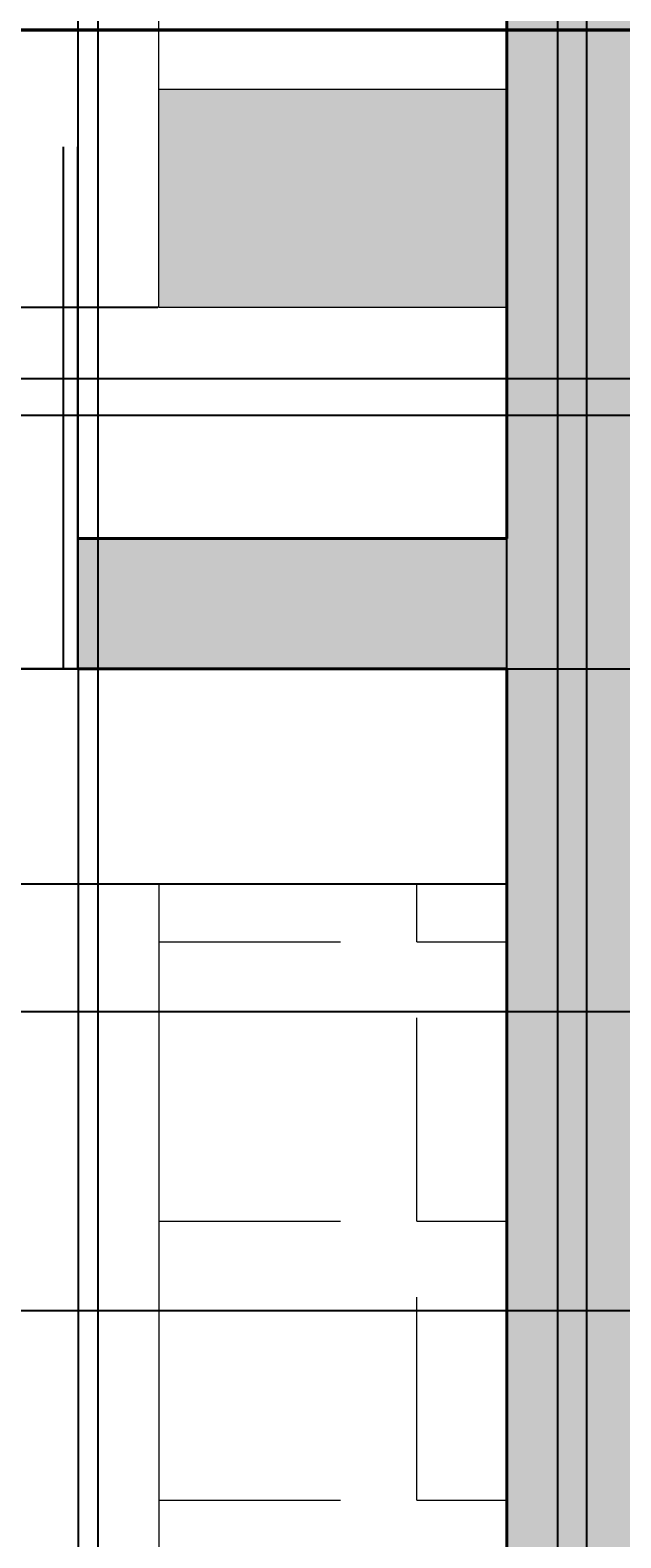
# Model space of a CAD drawing. Units: inches. Extents: x 818 to 1898, y 976 to 2364.
# Tile 25 of 96: x 1398 to 1439, y 1441 to 1545. Entities that reach past the tile are written whole.
import ezdxf

# ---------------------------------------------------------------- set-up
doc = ezdxf.new("R2010")
doc.units = ezdxf.units.IN
doc.header["$LTSCALE"] = 5
doc.header["$MEASUREMENT"] = 0
for name, color, linetype, lineweight in [('A-ANNO-DIMS', 2, 'Continuous', 18), ('A-DOOR', 3, 'Continuous', 25), ('A-FLOR-CASE', 8, 'Continuous', 18), ('A-FLOR-STRS', 7, 'Continuous', 25), ('A-FURN-PATT', 8, 'Continuous', 9), ('A-WALL', 7, 'Continuous', 40), ('C-PKNG', 8, 'Continuous', 18), ('C-PKNG-PATT', 9, 'Continuous', 9)]:
    doc.layers.add(name, color=color, linetype=linetype, lineweight=lineweight)
doc.layers.add('A-WALL-PATT', color=251, linetype='Continuous', lineweight=13, true_color=0x636466)
doc.styles.get("Standard").update_dxf_attribs({"font": 'arial.ttf'})
doc.dimstyles.get("Standard").update_dxf_attribs({"dimtxt": 0.18, "dimasz": 0.18, "dimexe": 0.18, "dimexo": 0.0625, "dimgap": 0.09, "dimtad": 0, "dimtih": 1, "dimtoh": 1, "dimdec": 4, "dimzin": 0, "dimdsep": 46, "dimtxsty": 'Standard', "dimcen": 0.09, "dimadec": 0, "dimazin": 0, "dimtfac": 1, "dimtdec": 4, "dimtofl": 0, "dimtmove": 0, "dimatfit": 3, "dimfxl": 1, "dimtolj": 1, "dimtzin": 0, "dimarcsym": 0})
pattern_1 = [(0, (0, 0), (0, 19.25), [14, -5.25]), (90, (0, 0), (-19.25, 1e-15), [14, -5.25])]

# ---------------------------------------------------------------- blocks, each defined once
blk = doc.blocks.new('*D61')
at = {"layer": 'A-ANNO-DIMS', "color": 0, "lineweight": -2, "ltscale": 5, "transparency": 16777216}
for p, q in [((1071.73, 1203.03), (1071.73, 2363.87)), ((1071.91, 2363.69), (1250.94, 2363.69)), ((1430.55, 2363.69), (1251.51, 2363.69)), ((1430.73, 1203.03), (1430.73, 2363.87))]:
    blk.add_line(p, q, dxfattribs=at)
at = {"layer": 'A-ANNO-DIMS', "color": 0, "ltscale": 5, "transparency": 16777216}
for points in [[(1071.91, 2363.72), (1071.91, 2363.66), (1071.73, 2363.69)], [(1430.55, 2363.72), (1430.55, 2363.66), (1430.73, 2363.69)]]:
    blk.add_solid(points, dxfattribs=at)
at = {"layer": 'Defpoints', "color": 0, "ltscale": 5, "transparency": 16777216}
for p in [(1430.73, 2363.69), (1071.73, 1202.96), (1430.73, 1202.96)]:
    blk.add_point(p, dxfattribs=at)
at = {"layer": 'A-ANNO-DIMS', "color": 0, "ltscale": 5, "transparency": 16777216, "insert": (1251.23, 2363.69), "char_height": 0.18, "attachment_point": 5}
blk.add_mtext('\\A1;359', dxfattribs=at)
blk = doc.blocks.new('*D64')
at = {"layer": 'A-ANNO-DIMS', "color": 0, "lineweight": -2, "ltscale": 5, "transparency": 16777216}
for p, q in [((1197.73, 1501.14), (1197.73, 2363.87)), ((1197.91, 2363.69), (1313.93, 2363.69)), ((1430.55, 2363.69), (1314.52, 2363.69)), ((1430.73, 1501.14), (1430.73, 2363.87))]:
    blk.add_line(p, q, dxfattribs=at)
at = {"layer": 'A-ANNO-DIMS', "color": 0, "ltscale": 5, "transparency": 16777216}
for points in [[(1197.91, 2363.72), (1197.91, 2363.66), (1197.73, 2363.69)], [(1430.55, 2363.72), (1430.55, 2363.66), (1430.73, 2363.69)]]:
    blk.add_solid(points, dxfattribs=at)
at = {"layer": 'Defpoints', "color": 0, "ltscale": 5, "transparency": 16777216}
for p in [(1430.73, 2363.69), (1197.73, 1501.08), (1430.73, 1501.08)]:
    blk.add_point(p, dxfattribs=at)
at = {"layer": 'A-ANNO-DIMS', "color": 0, "ltscale": 5, "transparency": 16777216, "insert": (1314.23, 2363.69), "char_height": 0.18, "attachment_point": 5}
blk.add_mtext('\\A1;233', dxfattribs=at)
blk = doc.blocks.new('*D99')
at = {"layer": 'A-ANNO-DIMS', "color": 0, "lineweight": -2, "ltscale": 5, "transparency": 16777216}
for p, q in [((1391.88, 1071.12), (1391.88, 2363.87)), ((1392.06, 2363.69), (1420.45, 2363.69)), ((1449.64, 2363.69), (1421.24, 2363.69)), ((1449.82, 1071.12), (1449.82, 2363.87))]:
    blk.add_line(p, q, dxfattribs=at)
at = {"layer": 'A-ANNO-DIMS', "color": 0, "ltscale": 5, "transparency": 16777216}
for points in [[(1392.06, 2363.72), (1392.06, 2363.66), (1391.88, 2363.69)], [(1449.64, 2363.72), (1449.64, 2363.66), (1449.82, 2363.69)]]:
    blk.add_solid(points, dxfattribs=at)
at = {"layer": 'Defpoints', "color": 0, "ltscale": 5, "transparency": 16777216}
for p in [(1449.82, 2363.69), (1391.88, 1071.06), (1449.82, 1071.06)]:
    blk.add_point(p, dxfattribs=at)
at = {"layer": 'A-ANNO-DIMS', "color": 0, "ltscale": 5, "transparency": 16777216, "insert": (1420.85, 2363.69), "char_height": 0.18, "attachment_point": 5}
blk.add_mtext('\\A1;57.94', dxfattribs=at)
blk = doc.blocks.new('*D116')
at = {"layer": 'A-ANNO-DIMS', "color": 0, "lineweight": -2, "ltscale": 5, "transparency": 16777216}
for p, q in [((1766.29, 1456.81), (818.03, 1456.81)), ((818.21, 1456.63), (818.21, 1417.41)), ((818.21, 1377.84), (818.21, 1417.05)), ((1766.29, 1377.66), (818.03, 1377.66))]:
    blk.add_line(p, q, dxfattribs=at)
at = {"layer": 'A-ANNO-DIMS', "color": 0, "ltscale": 5, "transparency": 16777216}
for points in [[(818.18, 1456.63), (818.24, 1456.63), (818.21, 1456.81)], [(818.18, 1377.84), (818.24, 1377.84), (818.21, 1377.66)]]:
    blk.add_solid(points, dxfattribs=at)
at = {"layer": 'Defpoints', "color": 0, "ltscale": 5, "transparency": 16777216}
for p in [(818.21, 1456.81), (1766.35, 1456.81), (1766.35, 1377.66)]:
    blk.add_point(p, dxfattribs=at)
at = {"layer": 'A-ANNO-DIMS', "color": 0, "ltscale": 5, "transparency": 16777216, "insert": (818.21, 1417.23), "char_height": 0.18, "attachment_point": 5}
blk.add_mtext('\\A1;79.15', dxfattribs=at)
blk = doc.blocks.new('*D117')
at = {"layer": 'A-ANNO-DIMS', "color": 0, "lineweight": -2, "ltscale": 5, "transparency": 16777216}
for p, q in [((1766.29, 1545.18), (818.03, 1545.18)), ((818.21, 1545), (818.21, 1501.18)), ((818.21, 1456.99), (818.21, 1500.81)), ((1766.29, 1456.81), (818.03, 1456.81))]:
    blk.add_line(p, q, dxfattribs=at)
at = {"layer": 'A-ANNO-DIMS', "color": 0, "ltscale": 5, "transparency": 16777216}
for points in [[(818.18, 1545), (818.24, 1545), (818.21, 1545.18)], [(818.18, 1456.99), (818.24, 1456.99), (818.21, 1456.81)]]:
    blk.add_solid(points, dxfattribs=at)
at = {"layer": 'Defpoints', "color": 0, "ltscale": 5, "transparency": 16777216}
for p in [(818.21, 1545.18), (1766.35, 1545.18), (1766.35, 1456.81)]:
    blk.add_point(p, dxfattribs=at)
at = {"layer": 'A-ANNO-DIMS', "color": 0, "ltscale": 5, "transparency": 16777216, "insert": (818.21, 1501), "char_height": 0.18, "attachment_point": 5}
blk.add_mtext('\\A1;88.37', dxfattribs=at)
blk = doc.blocks.new('*D159')
at = {"layer": 'A-ANNO-DIMS', "color": 0, "lineweight": -2, "ltscale": 5, "transparency": 16777216}
for p, q in [((1206.73, 1687.02), (1206.73, 975.66)), ((1463.73, 1687.02), (1463.73, 975.66)), ((1206.91, 975.84), (1334.93, 975.84)), ((1463.55, 975.84), (1335.52, 975.84))]:
    blk.add_line(p, q, dxfattribs=at)
at = {"layer": 'A-ANNO-DIMS', "color": 0, "ltscale": 5, "transparency": 16777216}
for points in [[(1206.91, 975.87), (1206.91, 975.81), (1206.73, 975.84)], [(1463.55, 975.87), (1463.55, 975.81), (1463.73, 975.84)]]:
    blk.add_solid(points, dxfattribs=at)
at = {"layer": 'Defpoints', "color": 0, "ltscale": 5, "transparency": 16777216}
for p in [(1206.73, 1687.08), (1463.73, 1687.08), (1463.73, 975.84)]:
    blk.add_point(p, dxfattribs=at)
at = {"layer": 'A-ANNO-DIMS', "color": 0, "ltscale": 5, "transparency": 16777216, "insert": (1335.23, 975.84), "char_height": 0.18, "attachment_point": 5}
blk.add_mtext('\\A1;257', dxfattribs=at)
blk = doc.blocks.new('*D163')
at = {"layer": 'A-ANNO-DIMS', "color": 0, "lineweight": -2, "ltscale": 5, "transparency": 16777216}
for p, q in [((1365.15, 1501.02), (1365.15, 975.66)), ((1401.15, 1501.02), (1401.15, 975.66)), ((1365.33, 975.84), (1382.93, 975.84)), ((1400.97, 975.84), (1383.37, 975.84))]:
    blk.add_line(p, q, dxfattribs=at)
at = {"layer": 'A-ANNO-DIMS', "color": 0, "ltscale": 5, "transparency": 16777216}
for points in [[(1365.33, 975.87), (1365.33, 975.81), (1365.15, 975.84)], [(1400.97, 975.87), (1400.97, 975.81), (1401.15, 975.84)]]:
    blk.add_solid(points, dxfattribs=at)
at = {"layer": 'Defpoints', "color": 0, "ltscale": 5, "transparency": 16777216}
for p in [(1365.15, 1501.08), (1401.15, 1501.08), (1401.15, 975.84)]:
    blk.add_point(p, dxfattribs=at)
at = {"layer": 'A-ANNO-DIMS', "color": 0, "ltscale": 5, "transparency": 16777216, "insert": (1383.15, 975.84), "char_height": 0.18, "attachment_point": 5}
blk.add_mtext('\\A1;36', dxfattribs=at)
blk = doc.blocks.new('*D166')
at = {"layer": 'A-ANNO-DIMS', "color": 0, "lineweight": -2, "ltscale": 5, "transparency": 16777216}
for p, q in [((1401.15, 1510.14), (1401.15, 2363.87)), ((1401.33, 2363.69), (1415.54, 2363.69)), ((1430.55, 2363.69), (1416.33, 2363.69)), ((1430.73, 1510.14), (1430.73, 2363.87))]:
    blk.add_line(p, q, dxfattribs=at)
at = {"layer": 'A-ANNO-DIMS', "color": 0, "ltscale": 5, "transparency": 16777216}
for points in [[(1401.33, 2363.72), (1401.33, 2363.66), (1401.15, 2363.69)], [(1430.55, 2363.72), (1430.55, 2363.66), (1430.73, 2363.69)]]:
    blk.add_solid(points, dxfattribs=at)
at = {"layer": 'Defpoints', "color": 0, "ltscale": 5, "transparency": 16777216}
for p in [(1430.73, 2363.69), (1401.15, 1510.08), (1430.73, 1510.08)]:
    blk.add_point(p, dxfattribs=at)
at = {"layer": 'A-ANNO-DIMS', "color": 0, "ltscale": 5, "transparency": 16777216, "insert": (1415.94, 2363.69), "char_height": 0.18, "attachment_point": 5}
blk.add_mtext('\\A1;29.58', dxfattribs=at)
blk = doc.blocks.new('*D167')
at = {"layer": 'A-ANNO-DIMS', "color": 0, "lineweight": -2, "ltscale": 5, "transparency": 16777216}
for p, q in [((1345.97, 1486.18), (1345.97, 975.66)), ((1430.73, 1486.18), (1430.73, 975.66)), ((1346.15, 975.84), (1387.95, 975.84)), ((1430.55, 975.84), (1388.74, 975.84))]:
    blk.add_line(p, q, dxfattribs=at)
at = {"layer": 'A-ANNO-DIMS', "color": 0, "ltscale": 5, "transparency": 16777216}
for points in [[(1346.15, 975.87), (1346.15, 975.81), (1345.97, 975.84)], [(1430.55, 975.87), (1430.55, 975.81), (1430.73, 975.84)]]:
    blk.add_solid(points, dxfattribs=at)
at = {"layer": 'Defpoints', "color": 0, "ltscale": 5, "transparency": 16777216}
for p in [(1345.97, 1486.24), (1430.73, 1486.24), (1430.73, 975.84)]:
    blk.add_point(p, dxfattribs=at)
at = {"layer": 'A-ANNO-DIMS', "color": 0, "ltscale": 5, "transparency": 16777216, "insert": (1388.35, 975.84), "char_height": 0.18, "attachment_point": 5}
blk.add_mtext('\\A1;84.76', dxfattribs=at)
blk = doc.blocks.new('*D168')
at = {"layer": 'A-ANNO-DIMS', "color": 0, "lineweight": -2, "ltscale": 5, "transparency": 16777216}
for p, q in [((1430.66, 1501.08), (818.03, 1501.08)), ((818.21, 1500.9), (818.21, 1493.84)), ((818.21, 1486.42), (818.21, 1493.48)), ((1430.66, 1486.24), (818.03, 1486.24))]:
    blk.add_line(p, q, dxfattribs=at)
at = {"layer": 'A-ANNO-DIMS', "color": 0, "ltscale": 5, "transparency": 16777216}
for points in [[(818.18, 1500.9), (818.24, 1500.9), (818.21, 1501.08)], [(818.18, 1486.42), (818.24, 1486.42), (818.21, 1486.24)]]:
    blk.add_solid(points, dxfattribs=at)
at = {"layer": 'Defpoints', "color": 0, "ltscale": 5, "transparency": 16777216}
for p in [(818.21, 1501.08), (1430.73, 1501.08), (1430.73, 1486.24)]:
    blk.add_point(p, dxfattribs=at)
at = {"layer": 'A-ANNO-DIMS', "color": 0, "ltscale": 5, "transparency": 16777216, "insert": (818.21, 1493.66), "char_height": 0.18, "attachment_point": 5}
blk.add_mtext('\\A1;14.84', dxfattribs=at)
blk = doc.blocks.new('*D170')
at = {"layer": 'A-ANNO-DIMS', "color": 0, "lineweight": -2, "ltscale": 5, "transparency": 16777216}
for p, q in [((1430.79, 1600.08), (1897.92, 1600.08)), ((1897.74, 1599.9), (1897.74, 1550.76)), ((1897.74, 1501.26), (1897.74, 1550.4)), ((1430.79, 1501.08), (1897.92, 1501.08))]:
    blk.add_line(p, q, dxfattribs=at)
at = {"layer": 'A-ANNO-DIMS', "color": 0, "ltscale": 5, "transparency": 16777216}
for points in [[(1897.71, 1599.9), (1897.77, 1599.9), (1897.74, 1600.08)], [(1897.71, 1501.26), (1897.77, 1501.26), (1897.74, 1501.08)]]:
    blk.add_solid(points, dxfattribs=at)
at = {"layer": 'Defpoints', "color": 0, "ltscale": 5, "transparency": 16777216}
for p in [(1430.73, 1600.08), (1897.74, 1600.08), (1430.73, 1501.08)]:
    blk.add_point(p, dxfattribs=at)
at = {"layer": 'A-ANNO-DIMS', "color": 0, "ltscale": 5, "transparency": 16777216, "insert": (1897.74, 1550.58), "char_height": 0.18, "attachment_point": 5}
blk.add_mtext('\\A1;99', dxfattribs=at)
blk = doc.blocks.new('*D187')
at = {"layer": 'A-ANNO-DIMS', "color": 0, "lineweight": -2, "ltscale": 5, "transparency": 16777216}
for p, q in [((1705.66, 1545.08), (818.03, 1545.08)), ((818.21, 1544.9), (818.21, 1533.26)), ((818.21, 1521.26), (818.21, 1532.9)), ((1705.66, 1521.08), (818.03, 1521.08))]:
    blk.add_line(p, q, dxfattribs=at)
at = {"layer": 'A-ANNO-DIMS', "color": 0, "ltscale": 5, "transparency": 16777216}
for points in [[(818.18, 1544.9), (818.24, 1544.9), (818.21, 1545.08)], [(818.18, 1521.26), (818.24, 1521.26), (818.21, 1521.08)]]:
    blk.add_solid(points, dxfattribs=at)
at = {"layer": 'Defpoints', "color": 0, "ltscale": 5, "transparency": 16777216}
for p in [(818.21, 1545.08), (1705.73, 1545.08), (1705.73, 1521.08)]:
    blk.add_point(p, dxfattribs=at)
at = {"layer": 'A-ANNO-DIMS', "color": 0, "ltscale": 5, "transparency": 16777216, "insert": (818.21, 1533.08), "char_height": 0.18, "attachment_point": 5}
blk.add_mtext('\\A1;24', dxfattribs=at)
blk = doc.blocks.new('*D191')
at = {"layer": 'A-ANNO-DIMS', "color": 0, "lineweight": -2, "ltscale": 5, "transparency": 16777216}
for p, q in [((1434.23, 1409.11), (1434.23, 2363.87)), ((1434.41, 2363.69), (1435.08, 2363.69)), ((1436.05, 2363.69), (1435.37, 2363.69)), ((1436.23, 1409.11), (1436.23, 2363.87))]:
    blk.add_line(p, q, dxfattribs=at)
at = {"layer": 'A-ANNO-DIMS', "color": 0, "ltscale": 5, "transparency": 16777216}
for points in [[(1434.41, 2363.72), (1434.41, 2363.66), (1434.23, 2363.69)], [(1436.05, 2363.72), (1436.05, 2363.66), (1436.23, 2363.69)]]:
    blk.add_solid(points, dxfattribs=at)
at = {"layer": 'Defpoints', "color": 0, "ltscale": 5, "transparency": 16777216}
for p in [(1436.23, 2363.69), (1434.23, 1409.05), (1436.23, 1409.05)]:
    blk.add_point(p, dxfattribs=at)
at = {"layer": 'A-ANNO-DIMS', "color": 0, "ltscale": 5, "transparency": 16777216, "insert": (1435.23, 2363.69), "char_height": 0.18, "attachment_point": 5}
blk.add_mtext('\\A1;2', dxfattribs=at)
blk = doc.blocks.new('*D198')
at = {"layer": 'A-ANNO-DIMS', "color": 0, "lineweight": -2, "ltscale": 5, "transparency": 16777216}
for p, q in [((1741.84, 1545.02), (1741.84, 975.66)), ((1430.73, 1346.02), (1430.73, 975.66)), ((1430.91, 975.84), (1585.91, 975.84)), ((1741.66, 975.84), (1586.66, 975.84))]:
    blk.add_line(p, q, dxfattribs=at)
at = {"layer": 'A-ANNO-DIMS', "color": 0, "ltscale": 5, "transparency": 16777216}
for points in [[(1430.91, 975.87), (1430.91, 975.81), (1430.73, 975.84)], [(1741.66, 975.87), (1741.66, 975.81), (1741.84, 975.84)]]:
    blk.add_solid(points, dxfattribs=at)
at = {"layer": 'Defpoints', "color": 0, "ltscale": 5, "transparency": 16777216}
for p in [(1741.84, 1545.08), (1430.73, 1346.08), (1741.84, 975.84)]:
    blk.add_point(p, dxfattribs=at)
at = {"layer": 'A-ANNO-DIMS', "color": 0, "ltscale": 5, "transparency": 16777216, "insert": (1586.28, 975.84), "char_height": 0.18, "attachment_point": 5}
blk.add_mtext('\\A1;311.1', dxfattribs=at)
blk = doc.blocks.new('*D201')
at = {"layer": 'A-ANNO-DIMS', "color": 0, "lineweight": -2, "ltscale": 5, "transparency": 16777216}
for p, q in [((1678.27, 1518.56), (818.03, 1518.56)), ((818.21, 1518.38), (818.21, 1498.18)), ((818.21, 1477.61), (818.21, 1497.81)), ((1678.27, 1477.43), (818.03, 1477.43))]:
    blk.add_line(p, q, dxfattribs=at)
at = {"layer": 'A-ANNO-DIMS', "color": 0, "ltscale": 5, "transparency": 16777216}
for points in [[(818.18, 1518.38), (818.24, 1518.38), (818.21, 1518.56)], [(818.18, 1477.61), (818.24, 1477.61), (818.21, 1477.43)]]:
    blk.add_solid(points, dxfattribs=at)
at = {"layer": 'Defpoints', "color": 0, "ltscale": 5, "transparency": 16777216}
for p in [(818.21, 1518.56), (1678.33, 1518.56), (1678.33, 1477.43)]:
    blk.add_point(p, dxfattribs=at)
at = {"layer": 'A-ANNO-DIMS', "color": 0, "ltscale": 5, "transparency": 16777216, "insert": (818.21, 1497.99), "char_height": 0.18, "attachment_point": 5}
blk.add_mtext('\\A1;41.135', dxfattribs=at)
blk = doc.blocks.new('*D231')
at = {"layer": 'A-ANNO-DIMS', "color": 0, "lineweight": -2, "ltscale": 5, "transparency": 16777216}
for p, q in [((1303.93, 1952.98), (1303.93, 975.66)), ((1402.52, 1952.98), (1402.52, 975.66)), ((1304.11, 975.84), (1352.83, 975.84)), ((1402.34, 975.84), (1353.62, 975.84))]:
    blk.add_line(p, q, dxfattribs=at)
at = {"layer": 'A-ANNO-DIMS', "color": 0, "ltscale": 5, "transparency": 16777216}
for points in [[(1304.11, 975.87), (1304.11, 975.81), (1303.93, 975.84)], [(1402.34, 975.87), (1402.34, 975.81), (1402.52, 975.84)]]:
    blk.add_solid(points, dxfattribs=at)
at = {"layer": 'Defpoints', "color": 0, "ltscale": 5, "transparency": 16777216}
for p in [(1303.93, 1953.04), (1402.52, 1953.04), (1402.52, 975.84)]:
    blk.add_point(p, dxfattribs=at)
at = {"layer": 'A-ANNO-DIMS', "color": 0, "ltscale": 5, "transparency": 16777216, "insert": (1353.22, 975.84), "char_height": 0.18, "attachment_point": 5}
blk.add_mtext('\\A1;98.59', dxfattribs=at)
blk = doc.blocks.new('*D272')
at = {"layer": 'A-ANNO-DIMS', "color": 0, "lineweight": -2, "ltscale": 5, "transparency": 16777216}
for p, q in [((1406.66, 1587.42), (818.03, 1587.42)), ((818.21, 1587.24), (818.21, 1556.89)), ((818.21, 1526.18), (818.21, 1556.52)), ((1406.66, 1526), (818.03, 1526))]:
    blk.add_line(p, q, dxfattribs=at)
at = {"layer": 'A-ANNO-DIMS', "color": 0, "ltscale": 5, "transparency": 16777216}
for points in [[(818.18, 1587.24), (818.24, 1587.24), (818.21, 1587.42)], [(818.18, 1526.18), (818.24, 1526.18), (818.21, 1526)]]:
    blk.add_solid(points, dxfattribs=at)
at = {"layer": 'Defpoints', "color": 0, "ltscale": 5, "transparency": 16777216}
for p in [(818.21, 1587.42), (1406.73, 1587.42), (1406.73, 1526)]:
    blk.add_point(p, dxfattribs=at)
at = {"layer": 'A-ANNO-DIMS', "color": 0, "ltscale": 5, "transparency": 16777216, "insert": (818.21, 1556.71), "char_height": 0.18, "attachment_point": 5}
blk.add_mtext('\\A1;61.42', dxfattribs=at)

msp = doc.modelspace()

# ---------------------------------------------------------------- hatches: boundary and pattern name
at = {"layer": 'A-FURN-PATT', "ltscale": 5}
h = msp.add_hatch(color=256, dxfattribs=at)
h.dxf.hatch_style = 1
h.paths.add_polyline_path([(1336.7936, 1953.0408), (1314.2595, 1953.0408), (1314.2595, 1941.0096), (1336.7936, 1941.0096)])
h.paths.add_polyline_path([(1338.9915, 1941.0096), (1336.7936, 1941.0096), (1336.7936, 1937.7177), (1314.2595, 1937.7177), (1314.2595, 1941.0096), (1310.9077, 1941.0096), (1310.9077, 1935.2252), (1338.9915, 1935.2252)])
h.paths.add_polyline_path([(1336.7936, 1941.0096), (1314.2595, 1941.0096), (1314.2595, 1937.7177), (1336.7936, 1937.7177)], flags=17)
h.paths.add_polyline_path([(1367.9307, 1959.6079), (1345.3966, 1959.6079), (1345.3966, 1941.0096), (1367.9307, 1941.0096)])
h.paths.add_polyline_path([(1398.8475, 1953.0408), (1376.3134, 1953.0408), (1376.3134, 1952.6393), (1390.1242, 1941.0096), (1398.8475, 1941.0096)])
h.paths.add_polyline_path([(1376.3134, 1952.6393), (1376.3134, 1941.0096), (1390.1242, 1941.0096)], flags=17)
h.paths.add_polyline_path([(1370.1286, 1941.0096), (1367.9307, 1941.0096), (1367.9307, 1937.7177), (1345.3966, 1937.7177), (1345.3966, 1941.0096), (1342.0448, 1941.0096), (1342.0448, 1935.2252), (1370.1286, 1935.2252)])
h.paths.add_polyline_path([(1367.9307, 1941.0096), (1345.3966, 1941.0096), (1345.3966, 1937.7177), (1367.9307, 1937.7177)], flags=17)
h.paths.add_polyline_path([(1390.1242, 1941.0096), (1376.3134, 1941.0096), (1376.3134, 1937.7177), (1394.0336, 1937.7177)], flags=17)
h.paths.add_polyline_path([(1394.0336, 1937.7177), (1376.3134, 1937.7177), (1376.3134, 1941.0096), (1372.9616, 1941.0096), (1372.9616, 1935.2252), (1396.9935, 1935.2252)])
h.paths.add_polyline_path([(1398.8475, 1941.0096), (1390.1242, 1941.0096), (1394.0336, 1937.7177), (1398.8475, 1937.7177)])
h.paths.add_polyline_path([(1401.0455, 1941.0096), (1398.8475, 1941.0096), (1398.8475, 1937.7177), (1394.0336, 1937.7177), (1396.9935, 1935.2252), (1401.0455, 1935.2252)])
h.paths.add_polyline_path([(1336.7936, 2020.4229), (1314.2595, 2020.4229), (1314.2595, 2008.3917), (1336.7936, 2008.3917)])
h.paths.add_polyline_path([(1336.7936, 2023.7149), (1314.2595, 2023.7149), (1314.2595, 2020.4229), (1336.7936, 2020.4229)], flags=17)
h.paths.add_polyline_path([(1338.9915, 2026.2074), (1310.9077, 2026.2074), (1310.9077, 2020.4229), (1314.2595, 2020.4229), (1314.2595, 2023.7149), (1336.7936, 2023.7149), (1336.7936, 2020.4229), (1338.9915, 2020.4229)])
h.paths.add_polyline_path([(1367.9307, 2023.7149), (1345.3966, 2023.7149), (1345.3966, 2020.4229), (1367.9307, 2020.4229)], flags=17)
h.paths.add_polyline_path([(1370.1286, 2026.2074), (1342.0448, 2026.2074), (1342.0448, 2020.4229), (1345.3966, 2020.4229), (1345.3966, 2023.7149), (1367.9307, 2023.7149), (1367.9307, 2020.4229), (1370.1286, 2020.4229)])
h.paths.add_polyline_path([(1367.9307, 2020.4229), (1345.3966, 2020.4229), (1345.3966, 2008.3917), (1367.9307, 2008.3917)])
h.paths.add_polyline_path([(1398.8475, 2020.4229), (1388.1824, 2020.4229), (1376.3134, 2010.4284), (1376.3134, 2008.3917), (1398.8475, 2008.3917)])
h.paths.add_polyline_path([(1392.0918, 2023.7149), (1376.3134, 2023.7149), (1376.3134, 2020.4229), (1388.1824, 2020.4229)], flags=17)
h.paths.add_polyline_path([(1388.1824, 2020.4229), (1376.3134, 2020.4229), (1376.3134, 2010.4284)], flags=17)
h.paths.add_polyline_path([(1395.0518, 2026.2074), (1372.9616, 2026.2074), (1372.9616, 2020.4229), (1376.3134, 2020.4229), (1376.3134, 2023.7149), (1392.0918, 2023.7149)])
h.paths.add_polyline_path([(1398.8475, 2023.7149), (1392.0918, 2023.7149), (1388.1824, 2020.4229), (1398.8475, 2020.4229)])
h.paths.add_polyline_path([(1401.0455, 2026.2074), (1395.0518, 2026.2074), (1392.0918, 2023.7149), (1398.8475, 2023.7149), (1398.8475, 2020.4229), (1401.0455, 2020.4229)])
h.paths.add_polyline_path([(1327.0339, 1897.8663), (1311.025, 1897.8663), (1311.025, 1876.0782), (1327.0339, 1876.0782)])
h.paths.add_polyline_path([(1377.7791, 1897.8663), (1359.9579, 1897.8663), (1359.9579, 1876.0782), (1377.7791, 1876.0782)])
h.paths.add_polyline_path([(1430.7251, 1541.0439), (1406.7251, 1541.0439), (1406.7251, 1525.9965), (1430.7251, 1525.9965)])
h.paths.add_polyline_path([(1430.7251, 1587.4164), (1406.7251, 1587.4164), (1406.7251, 1570.9187), (1430.7251, 1570.9187)])
at = {"layer": 'A-WALL-PATT', "ltscale": 5}
h = msp.add_hatch(color=256, dxfattribs=at)
h.dxf.hatch_style = 1
h.paths.add_polyline_path([(1206.7251, 1687.0782), (1206.7251, 1700.0782), (1197.7251, 1700.0782), (1197.7251, 1501.0782), (1206.7251, 1501.0782), (1206.7251, 1510.0782)])
h.paths.add_polyline_path([(1197.7251, 1590.7585), (1173.7252, 1590.7585), (1173.7252, 1586.7585), (1197.7251, 1586.7585)])
h.paths.add_polyline_path([(1197.7251, 1534.6024), (1173.7252, 1534.6024), (1173.7252, 1530.6024), (1197.7251, 1530.6024)])
h.paths.add_polyline_path([(1365.1463, 1510.0782), (1283.8183, 1510.0782), (1283.8183, 1501.0782), (1365.1463, 1501.0782)])
h.paths.add_polyline_path([(1439.7252, 1591.0782), (1441.7252, 1591.0782), (1441.7252, 1600.0782), (1430.7251, 1600.0782), (1430.7251, 1510.0782), (1406.7251, 1510.0782), (1401.1463, 1510.0782), (1401.1463, 1501.0782), (1430.7251, 1501.0782), (1430.7251, 1486.2383), (1430.7251, 1409.0522), (1439.7252, 1409.0522)])
at = {"layer": 'C-PKNG-PATT', "ltscale": 5}
h = msp.add_hatch(dxfattribs=at)
h.set_pattern_fill('ANGLE', color=256, scale=70)
h.set_pattern_definition(pattern_1)
h.paths.add_polyline_path([(1430.7251, 1211.9642), (1430.7251, 1486.2383), (1406.7251, 1486.2383), (1406.7251, 1235.9642), (1116.1882, 1235.9642), (1116.1882, 1485.2035), (1345.9651, 1485.2035), (1345.9651, 1501.0782), (1206.7251, 1501.0782), (1197.7251, 1501.0782), (1083.7252, 1501.0782), (1083.7252, 1485.2035), (1083.7252, 1211.9642)])
h = msp.add_hatch(dxfattribs=at)
h.set_pattern_fill('ANGLE', color=256, scale=70)
h.set_pattern_definition(pattern_1)
h.paths.add_polyline_path([(1116.1882, 1485.2035), (1345.9651, 1485.2035), (1345.9651, 1501.0782), (1206.7251, 1501.0782), (1197.7251, 1501.0782), (1083.7252, 1501.0782), (1083.7252, 1485.2035), (1083.7252, 1211.9642), (1430.7251, 1211.9642), (1430.7251, 1271.1621), (1430.7251, 1290.0782), (1430.7251, 1346.0782), (1430.7251, 1486.2383), (1406.7251, 1486.2383), (1406.7251, 1235.9642), (1116.1882, 1235.9642)])

# ---------------------------------------------------------------- linework, layer by layer
at = {"layer": 'A-DOOR'}
for p, q in [((1400.1463, 1501.0782), (1400.1463, 1537.0782)), ((1401.1463, 1501.0782), (1401.1463, 1537.0782)), ((1401.1463, 1510.0782), (1401.1463, 1501.0782))]:
    msp.add_line(p, q, dxfattribs=at)
at = {"layer": 'A-FLOR-CASE'}
for p, q in [((1406.7251, 1525.9965), (1406.7251, 1587.4164)), ((1430.7251, 1525.9965), (1406.7251, 1525.9965)), ((1430.7251, 1510.0782), (1406.7251, 1510.0782))]:
    msp.add_line(p, q, dxfattribs=at)
msp.add_lwpolyline([(1406.7251, 1570.9187), (1430.7251, 1570.9187), (1430.7251, 1541.0439), (1406.7251, 1541.0439)], close=True, dxfattribs=at)
at = {"layer": 'A-FLOR-STRS'}
msp.add_lwpolyline([(1345.9651, 1501.0782), (1430.7251, 1501.0782), (1430.7251, 1486.2383), (1345.9651, 1486.2383)], close=True, dxfattribs=at)
at = {"layer": 'A-WALL'}
for p, q in [((1430.7251, 1600.0782), (1430.7251, 1510.0782)), ((1401.1463, 1510.0782), (1430.7251, 1510.0782)), ((1401.1463, 1501.0782), (1430.7251, 1501.0782)), ((1430.7251, 1501.0782), (1430.7251, 1346.0782))]:
    msp.add_line(p, q, dxfattribs=at)
at = {"layer": 'C-PKNG'}
msp.add_line((1406.7251, 1486.2383), (1406.7251, 1235.9642), dxfattribs=at)

# ---------------------------------------------------------------- dimensions: what is measured, and where the dimension line sits
at = {"layer": 'A-ANNO-DIMS', "ltscale": 5}
for base, p1, p2, override, picture, middle in [((1430.7251, 2363.6929), (1071.7251, 1202.9642), (1430.7251, 1202.9642), {"dimdec": 0, "dimlfac": 1, "dimrnd": 0, "dimzin": 0, "dimdsep": 46, "dimlunit": 2}, '*D61', (1251.2251, 2363.6929)), ((1430.7251, 2363.6929), (1197.7251, 1501.0782), (1430.7251, 1501.0782), {"dimdec": 0, "dimlfac": 1, "dimrnd": 0, "dimzin": 0, "dimdsep": 46, "dimlunit": 2}, '*D64', (1314.2251, 2363.6929)), ((1449.8196, 2363.6929), (1391.8757, 1071.0552), (1449.8196, 1071.0552), {"dimdec": 2, "dimlfac": 1, "dimrnd": 0, "dimzin": 0, "dimdsep": 46, "dimlunit": 2}, '*D99', (1420.8477, 2363.6929)), ((1430.7251, 2363.6929), (1401.1463, 1510.0782), (1430.7251, 1510.0782), {"dimdec": 2, "dimlfac": 1, "dimrnd": 0, "dimzin": 0, "dimdsep": 46, "dimlunit": 2}, '*D166', (1415.9357, 2363.6929)), ((1436.2251, 2363.6929), (1434.2251, 1409.0522), (1436.2251, 1409.0522), {"dimdec": 0, "dimlfac": 1, "dimrnd": 0, "dimzin": 0, "dimdsep": 46, "dimlunit": 2}, '*D191', (1435.2251, 2363.6929)), ((1402.518, 975.8433), (1303.9314, 1953.0408), (1402.518, 1953.0408), {"dimdec": 2, "dimlfac": 1, "dimrnd": 0, "dimzin": 0, "dimdsep": 46, "dimlunit": 2}, '*D231', (1353.2247, 975.8433)), ((1463.7251, 975.8433), (1206.7251, 1687.0782), (1463.7251, 1687.0782), {"dimdec": 0, "dimlfac": 1, "dimrnd": 0, "dimzin": 0, "dimdsep": 46, "dimlunit": 2}, '*D159', (1335.2251, 975.8433)), ((1741.8409, 975.8433), (1430.7251, 1346.0782), (1741.8409, 1545.0782), {"dimdec": 1, "dimlfac": 1, "dimrnd": 0, "dimzin": 0, "dimdsep": 46, "dimlunit": 2}, '*D198', (1586.283, 975.8433)), ((1401.1463, 975.8433), (1365.1463, 1501.0782), (1401.1463, 1501.0782), {"dimdec": 0, "dimlfac": 1, "dimrnd": 0, "dimzin": 0, "dimdsep": 46, "dimlunit": 2}, '*D163', (1383.1463, 975.8433)), ((1430.7251, 975.8433), (1345.9651, 1486.2383), (1430.7251, 1486.2383), {"dimdec": 2, "dimlfac": 1, "dimrnd": 0, "dimzin": 0, "dimdsep": 46, "dimlunit": 2}, '*D167', (1388.3451, 975.8433))]:
    dim = msp.add_linear_dim(base=base, p1=p1, p2=p2, dimstyle='Standard', override=override, dxfattribs=at)
    dim.commit()
    dim.dimension.update_dxf_attribs({"geometry": picture, "text_midpoint": middle})
for base, p1, p2, override, picture, middle in [((1897.736, 1600.0782), (1430.7251, 1501.0782), (1430.7251, 1600.0782), {"dimdec": 0, "dimlfac": 1, "dimrnd": 0, "dimzin": 0, "dimdsep": 46, "dimlunit": 2}, '*D170', (1897.736, 1550.5782)), ((818.2059, 1587.4164), (1406.7251, 1525.9965), (1406.7251, 1587.4164), {"dimdec": 2, "dimlfac": 1, "dimrnd": 0, "dimzin": 0, "dimdsep": 46, "dimlunit": 2}, '*D272', (818.2059, 1556.7064)), ((818.2059, 1545.1827), (1766.3524, 1456.8088), (1766.3524, 1545.1827), {"dimdec": 2, "dimlfac": 1, "dimrnd": 0, "dimzin": 0, "dimdsep": 46, "dimlunit": 2}, '*D117', (818.2059, 1500.9957)), ((818.2059, 1545.0782), (1705.7251, 1521.0782), (1705.7251, 1545.0782), {"dimdec": 0, "dimlfac": 1, "dimrnd": 0, "dimzin": 0, "dimdsep": 46, "dimlunit": 2}, '*D187', (818.2059, 1533.0782)), ((818.2059, 1518.5611), (1678.3302, 1477.4261), (1678.3302, 1518.5611), {"dimdec": 3, "dimlfac": 1, "dimrnd": 0, "dimzin": 0, "dimdsep": 46, "dimlunit": 2}, '*D201', (818.2059, 1497.9936)), ((818.2059, 1501.0782), (1430.7251, 1486.2383), (1430.7251, 1501.0782), {"dimdec": 2, "dimlfac": 1, "dimrnd": 0, "dimzin": 0, "dimdsep": 46, "dimlunit": 2}, '*D168', (818.2059, 1493.6583)), ((818.2059, 1456.8088), (1766.3524, 1377.6564), (1766.3524, 1456.8088), {"dimdec": 2, "dimlfac": 1, "dimrnd": 0, "dimzin": 0, "dimdsep": 46, "dimlunit": 2}, '*D116', (818.2059, 1417.2326))]:
    dim = msp.add_linear_dim(base=base, p1=p1, p2=p2, angle=90, dimstyle='Standard', override=override, dxfattribs=at)
    dim.commit()
    dim.dimension.update_dxf_attribs({"geometry": picture, "text_midpoint": middle})

doc.saveas('drawing.dxf')
